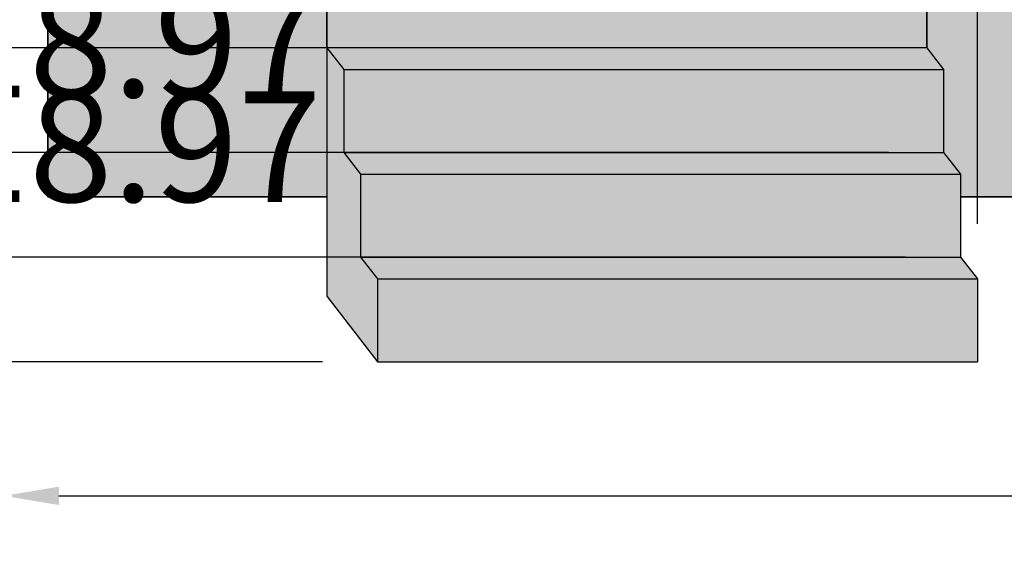
# Model space of a CAD drawing. Units: millimetres. Extents: x 130 to 1021, y 147 to 699.
# Tile 2 of 40: x 302 to 481, y 147 to 246. Entities that reach past the tile are written whole.
import ezdxf

# ---------------------------------------------------------------- set-up
doc = ezdxf.new("R2010")
doc.units = ezdxf.units.MM
doc.header["$MEASUREMENT"] = 0
for name, color, linetype, lineweight in [('A-ANNO-DIMS', 2, 'Continuous', 18), ('A-ELEV', 7, 'Continuous', 35), ('A-ELEV-PATT', 9, 'Continuous', 13), ('A-FLOR-STRS', 2, 'Continuous', 25)]:
    doc.layers.add(name, color=color, linetype=linetype, lineweight=lineweight)
doc.styles.get("Standard").update_dxf_attribs({"font": 'arial.ttf'})
doc.dimstyles.get("Standard").update_dxf_attribs({"dimtxt": 20, "dimasz": 10, "dimexe": 10, "dimexo": 10, "dimgap": 5, "dimtad": 0, "dimtih": 1, "dimtoh": 1, "dimdec": 0, "dimzin": 0, "dimdsep": 46, "dimtxsty": 'Standard', "dimcen": 5, "dimadec": 0, "dimazin": 0, "dimtfac": 1, "dimtdec": 0, "dimtofl": 0, "dimtmove": 0, "dimatfit": 3, "dimfxl": 1, "dimtolj": 1, "dimtzin": 0, "dimarcsym": 0})

# ---------------------------------------------------------------- blocks, each defined once
blk = doc.blocks.new('*D10')
at = {"layer": 'A-ANNO-DIMS', "color": 0, "lineweight": -2, "transparency": 16777216}
for p, q in [((440.89, 273.72), (430.89, 273.71)), ((473.57, 273.75), (483.57, 273.75)), ((450.9, 267.56), (450.9, 263.73)), ((463.58, 267.57), (463.58, 263.74))]:
    blk.add_line(p, q, dxfattribs=at)
at = {"layer": 'A-ANNO-DIMS', "color": 0, "transparency": 16777216}
for points in [[(440.89, 275.38), (440.89, 272.05), (450.89, 273.73)], [(473.57, 275.41), (473.58, 272.08), (463.57, 273.74)]]:
    blk.add_solid(points, dxfattribs=at)
at = {"layer": 'Defpoints', "color": 0, "transparency": 16777216}
for p in [(450.89, 277.56), (463.57, 277.57), (463.57, 273.74)]:
    blk.add_point(p, dxfattribs=at)
at = {"layer": 'A-ANNO-DIMS', "color": 0, "transparency": 16777216, "insert": (536.31, 273.75), "char_height": 20, "attachment_point": 5}
blk.add_mtext('\\A1;13 TYP.', dxfattribs=at)
blk = doc.blocks.new('*D11')
at = {"layer": 'A-ANNO-DIMS', "color": 0, "lineweight": -2, "transparency": 16777216}
for p, q in [((737.37, 648.7), (737.37, 149.74)), ((299.37, 566.95), (299.37, 149.74)), ((309.37, 159.74), (490.86, 159.74)), ((727.37, 159.74), (545.89, 159.74))]:
    blk.add_line(p, q, dxfattribs=at)
at = {"layer": 'A-ANNO-DIMS', "color": 0, "transparency": 16777216}
for points in [[(309.37, 161.41), (309.37, 158.07), (299.37, 159.74)], [(727.37, 161.41), (727.37, 158.07), (737.37, 159.74)]]:
    blk.add_solid(points, dxfattribs=at)
at = {"layer": 'Defpoints', "color": 0, "transparency": 16777216}
for p in [(737.37, 658.7), (299.37, 576.95), (737.37, 159.74)]:
    blk.add_point(p, dxfattribs=at)
at = {"layer": 'A-ANNO-DIMS', "color": 0, "transparency": 16777216, "insert": (518.37, 159.74), "char_height": 20, "attachment_point": 5}
blk.add_mtext('\\A1;438', dxfattribs=at)
blk = doc.blocks.new('*D12')
at = {"layer": 'A-ANNO-DIMS', "color": 0, "lineweight": -2, "transparency": 16777216}
for p, q in [((477.37, 661.95), (265.07, 661.95)), ((275.07, 651.95), (275.07, 438.2)), ((275.07, 194.04), (275.07, 407.78)), ((357.16, 184.04), (265.07, 184.04))]:
    blk.add_line(p, q, dxfattribs=at)
at = {"layer": 'A-ANNO-DIMS', "color": 0, "transparency": 16777216}
for points in [[(273.41, 651.95), (276.74, 651.95), (275.07, 661.95)], [(273.41, 194.04), (276.74, 194.04), (275.07, 184.04)]]:
    blk.add_solid(points, dxfattribs=at)
at = {"layer": 'Defpoints', "color": 0, "transparency": 16777216}
for p in [(275.07, 661.95), (487.37, 661.95), (367.16, 184.04)]:
    blk.add_point(p, dxfattribs=at)
at = {"layer": 'A-ANNO-DIMS', "color": 0, "transparency": 16777216, "insert": (275.07, 422.99), "char_height": 20, "attachment_point": 5}
blk.add_mtext('\\A1;477.9', dxfattribs=at)
blk = doc.blocks.new('*D23')
at = {"layer": 'A-ANNO-DIMS', "color": 0, "lineweight": -2, "transparency": 16777216}
for p, q in [((466.77, 403.95), (466.77, 696.25)), ((475.99, 209.04), (475.99, 696.25)), ((456.77, 686.25), (446.77, 686.25)), ((485.99, 686.25), (495.99, 686.25))]:
    blk.add_line(p, q, dxfattribs=at)
at = {"layer": 'A-ANNO-DIMS', "color": 0, "transparency": 16777216}
for points in [[(456.77, 687.91), (456.77, 684.58), (466.77, 686.25)], [(485.99, 687.91), (485.99, 684.58), (475.99, 686.25)]]:
    blk.add_solid(points, dxfattribs=at)
at = {"layer": 'Defpoints', "color": 0, "transparency": 16777216}
for p in [(475.99, 686.25), (466.77, 393.95), (475.99, 199.04)]:
    blk.add_point(p, dxfattribs=at)
at = {"layer": 'A-ANNO-DIMS', "color": 0, "transparency": 16777216, "insert": (534.63, 686.25), "char_height": 20, "attachment_point": 5}
blk.add_mtext('\\A1;9.222', dxfattribs=at)
blk = doc.blocks.new('*D24')
at = {"layer": 'A-ANNO-DIMS', "color": 0, "lineweight": -2, "transparency": 16777216}
for p, q in [((475.99, 209.04), (475.99, 696.25)), ((487.37, 671.95), (487.37, 696.25)), ((465.99, 686.25), (455.99, 686.25)), ((497.37, 686.25), (507.37, 686.25))]:
    blk.add_line(p, q, dxfattribs=at)
at = {"layer": 'A-ANNO-DIMS', "color": 0, "transparency": 16777216}
for points in [[(465.99, 687.91), (465.99, 684.58), (475.99, 686.25)], [(497.37, 687.91), (497.37, 684.58), (487.37, 686.25)]]:
    blk.add_solid(points, dxfattribs=at)
at = {"layer": 'Defpoints', "color": 0, "transparency": 16777216}
for p in [(487.37, 686.25), (487.37, 661.95), (475.99, 199.04)]:
    blk.add_point(p, dxfattribs=at)
at = {"layer": 'A-ANNO-DIMS', "color": 0, "transparency": 16777216, "insert": (553.02, 686.25), "char_height": 20, "attachment_point": 5}
blk.add_mtext('\\A1;11.385', dxfattribs=at)
blk = doc.blocks.new('*D33')
at = {"layer": 'A-ANNO-DIMS', "color": 0, "lineweight": -2, "transparency": 16777216}
for p, q in [((275.07, 213.01), (275.07, 223.01)), ((275.07, 223.01), (285.07, 223.01)), ((462.91, 203.01), (265.07, 203.01)), ((357.16, 184.04), (265.07, 184.04)), ((275.07, 174.04), (275.07, 164.04))]:
    blk.add_line(p, q, dxfattribs=at)
at = {"layer": 'A-ANNO-DIMS', "color": 0, "transparency": 16777216}
for points in [[(273.41, 213.01), (276.74, 213.01), (275.07, 203.01)], [(273.41, 174.04), (276.74, 174.04), (275.07, 184.04)]]:
    blk.add_solid(points, dxfattribs=at)
at = {"layer": 'Defpoints', "color": 0, "transparency": 16777216}
for p in [(275.07, 203.01), (472.91, 203.01), (367.16, 184.04)]:
    blk.add_point(p, dxfattribs=at)
at = {"layer": 'A-ANNO-DIMS', "color": 0, "transparency": 16777216, "insert": (322.88, 223.01), "char_height": 20, "attachment_point": 5}
blk.add_mtext('\\A1;18.97', dxfattribs=at)
blk = doc.blocks.new('*D34')
at = {"layer": 'A-ANNO-DIMS', "color": 0, "lineweight": -2, "transparency": 16777216}
for p, q in [((275.07, 231.98), (275.07, 241.98)), ((275.07, 241.98), (285.07, 241.98)), ((459.84, 221.98), (265.07, 221.98)), ((462.91, 203.01), (265.07, 203.01)), ((275.07, 193.01), (275.07, 183.01))]:
    blk.add_line(p, q, dxfattribs=at)
at = {"layer": 'A-ANNO-DIMS', "color": 0, "transparency": 16777216}
for points in [[(273.41, 231.98), (276.74, 231.98), (275.07, 221.98)], [(273.41, 193.01), (276.74, 193.01), (275.07, 203.01)]]:
    blk.add_solid(points, dxfattribs=at)
at = {"layer": 'Defpoints', "color": 0, "transparency": 16777216}
for p in [(275.07, 221.98), (469.84, 221.98), (472.91, 203.01)]:
    blk.add_point(p, dxfattribs=at)
at = {"layer": 'A-ANNO-DIMS', "color": 0, "transparency": 16777216, "insert": (322.88, 241.98), "char_height": 20, "attachment_point": 5}
blk.add_mtext('\\A1;18.97', dxfattribs=at)
blk = doc.blocks.new('*D35')
at = {"layer": 'A-ANNO-DIMS', "color": 0, "lineweight": -2, "transparency": 16777216}
for p, q in [((275.07, 250.95), (275.07, 260.95)), ((275.07, 260.95), (285.07, 260.95)), ((456.77, 240.95), (265.07, 240.95)), ((459.84, 221.98), (265.07, 221.98)), ((275.07, 211.98), (275.07, 201.98))]:
    blk.add_line(p, q, dxfattribs=at)
at = {"layer": 'A-ANNO-DIMS', "color": 0, "transparency": 16777216}
for points in [[(273.41, 250.95), (276.74, 250.95), (275.07, 240.95)], [(273.41, 211.98), (276.74, 211.98), (275.07, 221.98)]]:
    blk.add_solid(points, dxfattribs=at)
at = {"layer": 'Defpoints', "color": 0, "transparency": 16777216}
for p in [(275.07, 240.95), (466.77, 240.95), (469.84, 221.98)]:
    blk.add_point(p, dxfattribs=at)
at = {"layer": 'A-ANNO-DIMS', "color": 0, "transparency": 16777216, "insert": (322.88, 260.95), "char_height": 20, "attachment_point": 5}
blk.add_mtext('\\A1;18.97', dxfattribs=at)
blk = doc.blocks.new('*D36')
at = {"layer": 'A-ANNO-DIMS', "color": 0, "lineweight": -2, "transparency": 16777216}
for p, q in [((275.07, 270.95), (275.07, 280.95)), ((275.07, 280.95), (285.07, 280.95)), ((297.37, 260.95), (265.07, 260.95)), ((456.77, 240.95), (265.07, 240.95)), ((275.07, 230.95), (275.07, 220.95))]:
    blk.add_line(p, q, dxfattribs=at)
at = {"layer": 'A-ANNO-DIMS', "color": 0, "transparency": 16777216}
for points in [[(273.41, 270.95), (276.74, 270.95), (275.07, 260.95)], [(273.41, 230.95), (276.74, 230.95), (275.07, 240.95)]]:
    blk.add_solid(points, dxfattribs=at)
at = {"layer": 'Defpoints', "color": 0, "transparency": 16777216}
for p in [(275.07, 260.95), (307.37, 260.95), (466.77, 240.95)]:
    blk.add_point(p, dxfattribs=at)
at = {"layer": 'A-ANNO-DIMS', "color": 0, "transparency": 16777216, "insert": (304.53, 280.95), "char_height": 20, "attachment_point": 5}
blk.add_mtext('\\A1;20', dxfattribs=at)
blk = doc.blocks.new('*D37')
at = {"layer": 'A-ANNO-DIMS', "color": 0, "lineweight": -2, "transparency": 16777216}
for p, q in [((275.07, 283.95), (275.07, 293.95)), ((275.07, 293.95), (285.07, 293.95)), ((297.37, 273.95), (265.07, 273.95)), ((297.37, 260.95), (265.07, 260.95)), ((275.07, 250.95), (275.07, 240.95))]:
    blk.add_line(p, q, dxfattribs=at)
at = {"layer": 'A-ANNO-DIMS', "color": 0, "transparency": 16777216}
for points in [[(273.41, 283.95), (276.74, 283.95), (275.07, 273.95)], [(273.41, 250.95), (276.74, 250.95), (275.07, 260.95)]]:
    blk.add_solid(points, dxfattribs=at)
at = {"layer": 'Defpoints', "color": 0, "transparency": 16777216}
for p in [(275.07, 273.95), (307.37, 273.95), (307.37, 260.95)]:
    blk.add_point(p, dxfattribs=at)
at = {"layer": 'A-ANNO-DIMS', "color": 0, "transparency": 16777216, "insert": (303.46, 293.95), "char_height": 20, "attachment_point": 5}
blk.add_mtext('\\A1;13', dxfattribs=at)

msp = doc.modelspace()

# ---------------------------------------------------------------- hatches: boundary and pattern name
at = {"layer": 'A-ELEV-PATT'}
h = msp.add_hatch(color=256, dxfattribs=at)
h.dxf.hatch_style = 1
h.paths.add_polyline_path([(737.3738, 658.6988, 0.01359606), (632.4019, 661.9473), (607.3738, 661.9473), (487.3738, 661.9473), (487.3738, 649.9473), (607.3738, 649.9473), (632.3794, 649.9473, -0.01368411), (737.3738, 646.6784)])
h.paths.add_polyline_path([(732.3738, 643.9599, 0.01305286), (632.3738, 646.9473), (607.3738, 646.9473), (487.3738, 646.9473), (487.3738, 596.9473), (632.3738, 596.9473, -0.01305286), (732.3738, 593.9599)])
h.paths.add_polyline_path([(737.3738, 593.6732, 0.01370629), (632.3738, 596.9473), (487.3738, 596.9473), (487.3738, 586.9473), (632.355, 586.9473, -0.01378075), (737.3738, 583.6559)])
h.paths.add_polyline_path([(447.3738, 646.9473), (307.3738, 646.9473), (302.3738, 646.9473), (302.3738, 634.9473), (447.3738, 634.9473)])
h.paths.add_polyline_path([(447.3738, 631.9473), (307.3738, 631.9473), (307.3738, 586.9473), (447.3738, 586.9473)])
h.paths.add_polyline_path([(447.3738, 586.9473), (307.3738, 586.9473), (302.3738, 586.9473), (302.3738, 576.9473), (447.3738, 576.9473)])
h.paths.add_polyline_path([(447.3738, 573.9473), (367.3738, 573.9473), (367.3738, 539.9473), (447.3738, 539.9473)])
h.paths.add_polyline_path([(447.3738, 537.9473), (367.3738, 537.9473), (367.3738, 507.9473), (400.392, 507.4253, -0.00172798), (401.3281, 507.6451, -0.52200255), (425.6117, 511.0391, -0.03918489), (447.3738, 510.4359), (447.3738, 510.7883)])
h.paths.add_polyline_path([(394.7238, 505.9473), (367.3738, 505.9473), (367.3738, 476.9473, -0.0146512), (375.8501, 480.2159), (376.1506, 499.2266, -0.03554194)])
h.paths.add_polyline_path([(632.3738, 583.9473), (552.3738, 583.9473), (552.3738, 550.9473), (632.3738, 550.9473)])
h.paths.add_polyline_path([(632.3738, 548.9473), (552.3738, 548.9473), (552.3738, 515.9473), (632.3738, 515.9473)])
h.paths.add_polyline_path([(632.3738, 513.9473), (552.3738, 513.9473), (552.3738, 476.9473), (632.3738, 476.9473)])
h.paths.add_polyline_path([(737.3738, 473.6903, 0.01363261), (632.3926, 476.9473), (552.3738, 476.9473), (487.3738, 476.9473), (487.3738, 466.9473), (632.3738, 466.9473, -0.01370629), (737.3738, 463.6732)])
h.paths.add_polyline_path([(732.3738, 460.9552, 0.01307409), (632.3681, 463.9473), (487.3738, 463.9473), (487.3738, 407.735, -0.00322862), (489.3544, 406.9473), (632.3926, 406.9473, -0.01298259), (732.3738, 403.9755)])
h.paths.add_polyline_path([(487.3738, 463.9473, 0.20132998), (367.3738, 463.9473), (367.3738, 407.735, -0.18820307), (487.3738, 407.735)])
h.paths.add_polyline_path([(367.3738, 476.9473), (367.3738, 466.9473, -0.20133085), (487.3738, 466.9473), (487.3738, 476.9473, 0.20132998)])
h.paths.add_polyline_path([(367.3738, 463.9473), (307.3738, 463.9473), (307.3738, 401.9473), (357.9413, 401.9473), (367.3738, 407.735)])
h.paths.add_polyline_path([(367.3738, 476.9473), (302.3738, 476.9473), (302.3738, 466.9473), (367.3738, 466.9473)])
h.paths.add_polyline_path([(632.8184, 366.9453), (552.3738, 366.9453), (552.3738, 393.9473), (632.8184, 393.9473)])
h.paths.add_polyline_path([(632.8184, 357.2114), (632.8184, 363.9453), (552.3738, 363.9453), (552.3738, 357.2114), (552.3738, 336.9453), (632.8184, 336.9453)])
h.paths.add_polyline_path([(632.8184, 333.9453), (552.3738, 333.9453), (552.3738, 306.9453), (632.8184, 306.9453)])
h.paths.add_polyline_path([(632.8184, 303.9453), (552.3738, 303.9453), (552.3738, 273.9473), (632.355, 273.9473, 0.00006077), (632.8184, 273.9491)])
h.paths.add_polyline_path([(737.3738, 403.6903, 0.01363261), (632.3926, 406.9473), (489.3544, 406.9473, 0.19154808), (367.3738, 407.735), (367.3738, 396.9473, -0.20133085), (487.3738, 396.9473), (632.3738, 396.9473, -0.01370629), (737.3738, 393.6732)])
h.paths.add_polyline_path([(357.9413, 401.9473), (307.3738, 401.9473), (307.3738, 391.9473), (357.9413, 391.9473)])
h.paths.add_polyline_path([(357.9413, 357.2114), (357.9413, 388.9473), (307.3738, 388.9473), (307.3738, 357.2114), (307.3738, 273.9473), (357.9413, 273.9473)])
h.paths.add_polyline_path([(732.3738, 263.93, -0.0130317), (632.3794, 260.9473), (466.7667, 260.9473), (466.7667, 240.9473), (469.8406, 236.978), (469.8406, 221.978), (472.9145, 218.0087), (472.9145, 213.9473), (607.3738, 213.9473), (732.3738, 213.9473)])
h.paths.add_polyline_path([(732.3738, 290.889), (722.479, 290.889), (722.479, 301.889), (732.3738, 301.889), (732.3738, 305.889), (722.479, 305.889), (722.479, 316.889), (732.3738, 316.889), (732.3738, 320.889), (722.479, 320.889), (722.479, 331.889), (732.3738, 331.889), (732.3738, 335.889), (722.479, 335.889), (722.479, 346.889), (732.3738, 346.889), (732.3738, 350.889), (722.479, 350.889), (722.479, 361.889), (732.3738, 361.889), (732.3738, 365.889), (722.479, 365.889), (722.479, 376.889), (732.3738, 376.889), (732.3738, 380.889), (722.479, 380.889), (722.479, 391.4848, 0.00052326), (718.479, 391.6843), (718.479, 380.889), (707.479, 380.889), (707.479, 392.1896, 0.00052307), (703.479, 392.3576), (703.479, 380.889), (692.479, 380.889), (692.479, 392.7765, 0.00052292), (688.479, 392.9131), (688.479, 380.889), (677.479, 380.889), (677.479, 393.2456, 0.00052279), (673.479, 393.3508), (673.479, 380.889), (662.479, 380.889), (662.479, 393.597, 0.0005227), (658.479, 393.6709), (658.479, 380.889), (647.479, 380.889), (647.479, 393.8308, 0.00052264), (643.479, 393.8732), (643.479, 380.889), (632.8184, 380.889), (632.8184, 376.889), (643.479, 376.889), (643.479, 365.889), (632.8184, 365.889), (632.8184, 361.889), (643.479, 361.889), (643.479, 350.889), (632.8184, 350.889), (632.8184, 346.889), (643.479, 346.889), (643.479, 335.889), (632.8184, 335.889), (632.8184, 331.889), (643.479, 331.889), (643.479, 320.889), (632.8184, 320.889), (632.8184, 316.889), (643.479, 316.889), (643.479, 305.889), (632.8184, 305.889), (632.8184, 301.889), (643.479, 301.889), (643.479, 290.889), (632.8184, 290.889), (632.8184, 286.889), (643.479, 286.889), (643.479, 274.0217, 0.00052456), (647.479, 274.0643), (647.479, 286.889), (658.479, 286.889), (658.479, 274.2248, 0.00052462), (662.479, 274.2989), (662.479, 286.889), (673.479, 286.889), (673.479, 274.546, 0.00052471), (677.479, 274.6516), (677.479, 286.889), (688.479, 286.889), (688.479, 274.9853, 0.00052484), (692.479, 275.1224), (692.479, 286.889), (703.479, 286.889), (703.479, 275.5429, 0.000525), (707.479, 275.7115), (707.479, 286.889), (718.479, 286.889), (718.479, 276.2187, 0.00052519), (722.479, 276.4189), (722.479, 286.889), (732.3738, 286.889)])
h.paths.add_polyline_path([(718.479, 290.889), (707.479, 290.889), (707.479, 301.889), (718.479, 301.889)], flags=16)
h.paths.add_polyline_path([(703.479, 290.889), (692.479, 290.889), (692.479, 301.889), (703.479, 301.889)], flags=16)
h.paths.add_polyline_path([(718.479, 305.889), (707.479, 305.889), (707.479, 316.889), (718.479, 316.889)], flags=16)
h.paths.add_polyline_path([(703.479, 305.889), (692.479, 305.889), (692.479, 316.889), (703.479, 316.889)], flags=16)
h.paths.add_polyline_path([(688.479, 290.889), (677.479, 290.889), (677.479, 301.889), (688.479, 301.889)], flags=16)
h.paths.add_polyline_path([(718.479, 320.889), (707.479, 320.889), (707.479, 331.889), (718.479, 331.889)], flags=16)
h.paths.add_polyline_path([(688.479, 305.889), (677.479, 305.889), (677.479, 316.889), (688.479, 316.889)], flags=16)
h.paths.add_polyline_path([(703.479, 320.889), (692.479, 320.889), (692.479, 331.889), (703.479, 331.889)], flags=16)
h.paths.add_polyline_path([(688.479, 320.889), (677.479, 320.889), (677.479, 331.889), (688.479, 331.889)], flags=16)
h.paths.add_polyline_path([(673.479, 290.889), (662.479, 290.889), (662.479, 301.889), (673.479, 301.889)], flags=16)
h.paths.add_polyline_path([(718.479, 335.889), (707.479, 335.889), (707.479, 346.889), (718.479, 346.889)], flags=16)
h.paths.add_polyline_path([(673.479, 305.889), (662.479, 305.889), (662.479, 316.889), (673.479, 316.889)], flags=16)
h.paths.add_polyline_path([(703.479, 335.889), (692.479, 335.889), (692.479, 346.889), (703.479, 346.889)], flags=16)
h.paths.add_polyline_path([(673.479, 320.889), (662.479, 320.889), (662.479, 331.889), (673.479, 331.889)], flags=16)
h.paths.add_polyline_path([(688.479, 335.889), (677.479, 335.889), (677.479, 346.889), (688.479, 346.889)], flags=16)
h.paths.add_polyline_path([(658.479, 290.889), (647.479, 290.889), (647.479, 301.889), (658.479, 301.889)], flags=16)
h.paths.add_polyline_path([(718.479, 350.889), (707.479, 350.889), (707.479, 361.889), (718.479, 361.889)], flags=16)
h.paths.add_polyline_path([(658.479, 305.889), (647.479, 305.889), (647.479, 316.889), (658.479, 316.889)], flags=16)
h.paths.add_polyline_path([(703.479, 350.889), (692.479, 350.889), (692.479, 361.889), (703.479, 361.889)], flags=16)
h.paths.add_polyline_path([(673.479, 335.889), (662.479, 335.889), (662.479, 346.889), (673.479, 346.889)], flags=16)
h.paths.add_polyline_path([(658.479, 320.889), (647.479, 320.889), (647.479, 331.889), (658.479, 331.889)], flags=16)
h.paths.add_polyline_path([(688.479, 350.889), (677.479, 350.889), (677.479, 361.889), (688.479, 361.889)], flags=16)
h.paths.add_polyline_path([(718.479, 365.889), (707.479, 365.889), (707.479, 376.889), (718.479, 376.889)], flags=16)
h.paths.add_polyline_path([(658.479, 335.889), (647.479, 335.889), (647.479, 346.889), (658.479, 346.889)], flags=16)
h.paths.add_polyline_path([(673.479, 350.889), (662.479, 350.889), (662.479, 361.889), (673.479, 361.889)], flags=16)
h.paths.add_polyline_path([(703.479, 365.889), (692.479, 365.889), (692.479, 376.889), (703.479, 376.889)], flags=16)
h.paths.add_polyline_path([(688.479, 365.889), (677.479, 365.889), (677.479, 376.889), (688.479, 376.889)], flags=16)
h.paths.add_polyline_path([(658.479, 350.889), (647.479, 350.889), (647.479, 361.889), (658.479, 361.889)], flags=16)
h.paths.add_polyline_path([(673.479, 365.889), (662.479, 365.889), (662.479, 376.889), (673.479, 376.889)], flags=16)
h.paths.add_polyline_path([(658.479, 365.889), (647.479, 365.889), (647.479, 376.889), (658.479, 376.889)], flags=16)
h.paths.add_polyline_path([(732.3738, 503.9786), (722.3392, 503.9786), (722.3392, 514.9786), (732.3738, 514.9786), (732.3738, 518.9786), (722.3392, 518.9786), (722.3392, 529.9786), (732.3738, 529.9786), (732.3738, 533.9786), (722.3392, 533.9786), (722.3392, 544.9786), (732.3738, 544.9786), (732.3738, 546.9473), (732.3738, 548.9786), (722.3392, 548.9786), (722.3392, 559.9786), (732.3738, 559.9786), (732.3738, 563.9786), (722.3392, 563.9786), (722.3392, 574.9786), (732.3738, 574.9786), (732.3738, 578.9786), (722.3392, 578.9786), (722.3392, 581.4789, 0.00052601), (718.3392, 581.6791), (718.3392, 578.9786), (707.3392, 578.9786), (707.3392, 582.1863, 0.00052582), (703.3392, 582.355), (703.3392, 578.9786), (692.3392, 578.9786), (692.3392, 582.7752, 0.00052566), (688.3392, 582.9123), (688.3392, 578.9786), (677.3392, 578.9786), (677.3392, 583.2457, 0.00052554), (673.3392, 583.3512), (673.3392, 578.9786), (662.3392, 578.9786), (662.3392, 583.5978, 0.00052545), (658.3392, 583.6718), (658.3392, 578.9786), (647.3392, 578.9786), (647.3392, 583.8317, 0.00052539), (643.3392, 583.8741), (643.3392, 578.9786), (632.3738, 578.9786), (632.3738, 574.9786), (643.3392, 574.9786), (643.3392, 563.9786), (632.3738, 563.9786), (632.3738, 559.9786), (643.3392, 559.9786), (643.3392, 548.9786), (632.3738, 548.9786), (632.3738, 544.9786), (643.3392, 544.9786), (643.3392, 533.9786), (632.3738, 533.9786), (632.3738, 529.9786), (643.3392, 529.9786), (643.3392, 518.9786), (632.3738, 518.9786), (632.3738, 515.9473), (632.3738, 514.9786), (643.3392, 514.9786), (643.3392, 503.9786), (632.3738, 503.9786), (632.3738, 499.9786), (643.3392, 499.9786), (643.3392, 488.9786), (632.3738, 488.9786), (632.3738, 484.9786), (643.3392, 484.9786), (643.3392, 476.8751, -0.00051911), (647.3392, 476.8332), (647.3392, 484.9786), (658.3392, 484.9786), (658.3392, 476.6752, -0.00051917), (662.3392, 476.6022), (662.3392, 484.9786), (673.3392, 484.9786), (673.3392, 476.3585, -0.00051926), (677.3392, 476.2543), (677.3392, 484.9786), (688.3392, 484.9786), (688.3392, 475.9248, -0.00051938), (692.3392, 475.7894), (692.3392, 484.9786), (703.3392, 484.9786), (703.3392, 475.3741, -0.00051953), (707.3392, 475.2075), (707.3392, 484.9786), (718.3392, 484.9786), (718.3392, 474.7064, -0.00051972), (722.3392, 474.5086), (722.3392, 484.9786), (732.3738, 484.9786), (732.3738, 488.9786), (722.3392, 488.9786), (722.3392, 499.9786), (732.3738, 499.9786)])
h.paths.add_polyline_path([(718.3392, 503.9786), (707.3392, 503.9786), (707.3392, 514.9786), (718.3392, 514.9786)], flags=16)
h.paths.add_polyline_path([(718.3392, 499.9786), (718.3392, 488.9786), (707.3392, 488.9786), (707.3392, 499.9786)], flags=16)
h.paths.add_polyline_path([(718.3392, 518.9786), (707.3392, 518.9786), (707.3392, 529.9786), (718.3392, 529.9786)], flags=16)
h.paths.add_polyline_path([(703.3392, 503.9786), (692.3392, 503.9786), (692.3392, 514.9786), (703.3392, 514.9786)], flags=16)
h.paths.add_polyline_path([(703.3392, 499.9786), (703.3392, 488.9786), (692.3392, 488.9786), (692.3392, 499.9786)], flags=16)
h.paths.add_polyline_path([(703.3392, 518.9786), (692.3392, 518.9786), (692.3392, 529.9786), (703.3392, 529.9786)], flags=16)
h.paths.add_polyline_path([(718.3392, 533.9786), (707.3392, 533.9786), (707.3392, 544.9786), (718.3392, 544.9786)], flags=16)
h.paths.add_polyline_path([(688.3392, 503.9786), (677.3392, 503.9786), (677.3392, 514.9786), (688.3392, 514.9786)], flags=16)
h.paths.add_polyline_path([(688.3392, 499.9786), (688.3392, 488.9786), (677.3392, 488.9786), (677.3392, 499.9786)], flags=16)
h.paths.add_polyline_path([(703.3392, 533.9786), (692.3392, 533.9786), (692.3392, 544.9786), (703.3392, 544.9786)], flags=16)
h.paths.add_polyline_path([(688.3392, 518.9786), (677.3392, 518.9786), (677.3392, 529.9786), (688.3392, 529.9786)], flags=16)
h.paths.add_polyline_path([(688.3392, 533.9786), (677.3392, 533.9786), (677.3392, 544.9786), (688.3392, 544.9786)], flags=16)
h.paths.add_polyline_path([(718.3392, 548.9786), (707.3392, 548.9786), (707.3392, 559.9786), (718.3392, 559.9786)], flags=16)
h.paths.add_polyline_path([(673.3392, 503.9786), (662.3392, 503.9786), (662.3392, 514.9786), (673.3392, 514.9786)], flags=16)
h.paths.add_polyline_path([(673.3392, 499.9786), (673.3392, 488.9786), (662.3392, 488.9786), (662.3392, 499.9786)], flags=16)
h.paths.add_polyline_path([(703.3392, 548.9786), (692.3392, 548.9786), (692.3392, 559.9786), (703.3392, 559.9786)], flags=16)
h.paths.add_polyline_path([(673.3392, 518.9786), (662.3392, 518.9786), (662.3392, 529.9786), (673.3392, 529.9786)], flags=16)
h.paths.add_polyline_path([(688.3392, 548.9786), (677.3392, 548.9786), (677.3392, 559.9786), (688.3392, 559.9786)], flags=16)
h.paths.add_polyline_path([(673.3392, 533.9786), (662.3392, 533.9786), (662.3392, 544.9786), (673.3392, 544.9786)], flags=16)
h.paths.add_polyline_path([(718.3392, 563.9786), (707.3392, 563.9786), (707.3392, 574.9786), (718.3392, 574.9786)], flags=16)
h.paths.add_polyline_path([(658.3392, 503.9786), (647.3392, 503.9786), (647.3392, 514.9786), (658.3392, 514.9786)], flags=16)
h.paths.add_polyline_path([(658.3392, 499.9786), (658.3392, 488.9786), (647.3392, 488.9786), (647.3392, 499.9786)], flags=16)
h.paths.add_polyline_path([(703.3392, 563.9786), (692.3392, 563.9786), (692.3392, 574.9786), (703.3392, 574.9786)], flags=16)
h.paths.add_polyline_path([(658.3392, 518.9786), (647.3392, 518.9786), (647.3392, 529.9786), (658.3392, 529.9786)], flags=16)
h.paths.add_polyline_path([(673.3392, 548.9786), (662.3392, 548.9786), (662.3392, 559.9786), (673.3392, 559.9786)], flags=16)
h.paths.add_polyline_path([(688.3392, 563.9786), (677.3392, 563.9786), (677.3392, 574.9786), (688.3392, 574.9786)], flags=16)
h.paths.add_polyline_path([(658.3392, 533.9786), (647.3392, 533.9786), (647.3392, 544.9786), (658.3392, 544.9786)], flags=16)
h.paths.add_polyline_path([(673.3392, 563.9786), (662.3392, 563.9786), (662.3392, 574.9786), (673.3392, 574.9786)], flags=16)
h.paths.add_polyline_path([(658.3392, 548.9786), (647.3392, 548.9786), (647.3392, 559.9786), (658.3392, 559.9786)], flags=16)
h.paths.add_polyline_path([(658.3392, 563.9786), (647.3392, 563.9786), (647.3392, 574.9786), (658.3392, 574.9786)], flags=16)
h = msp.add_hatch(color=256, dxfattribs=at)
h.dxf.hatch_style = 1
h.paths.add_polyline_path([(364.0891, 218.0087), (361.0152, 221.978), (361.0152, 236.978), (357.9413, 240.9473), (357.9413, 195.9473), (367.163, 184.0395), (367.163, 199.0395), (364.0891, 203.0087)])
h.paths.add_polyline_path([(502.3738, 537.2685), (502.3738, 513.9473), (547.7773, 513.9473), (547.7773, 537.2685)])
h.paths.add_polyline_path([(502.3738, 511.9473), (502.3738, 481.7432), (547.7773, 481.7432), (547.7773, 511.9473)])
h.paths.add_polyline_path([(327.3738, 529.7), (327.3738, 509.9473), (363.922, 509.9473), (363.922, 529.7)])
h.paths.add_polyline_path([(327.3738, 507.9473), (327.3738, 480.95), (363.922, 480.95), (363.922, 507.9473)])
h = msp.add_hatch(color=256, dxfattribs=at)
h.dxf.hatch_style = 1
h.paths.add_polyline_path([(357.9413, 240.9473), (357.9413, 260.9473), (307.3738, 260.9473), (307.3738, 213.9473), (357.9413, 213.9473)])
h.paths.add_polyline_path([(382.3738, 260.9473), (357.9413, 260.9473), (357.9413, 240.9473), (466.7667, 240.9473), (466.7667, 260.9473), (432.3738, 260.9473), (432.3738, 249.5473), (382.3738, 249.5473)])
h.paths.add_polyline_path([(357.9413, 273.9473), (307.3738, 273.9473), (307.3738, 263.9473), (357.9413, 263.9473)])
h.paths.add_polyline_path([(382.3738, 273.9473), (357.9413, 273.9473), (357.9413, 263.9473), (382.3738, 263.9473)])
h = msp.add_hatch(color=256, dxfattribs=at)
h.dxf.hatch_style = 1
h.paths.add_polyline_path([(466.7667, 240.9473), (357.9413, 240.9473), (361.0152, 236.978), (469.8406, 236.978)])
h.paths.add_polyline_path([(472.9145, 218.0087), (469.8406, 221.978), (361.0152, 221.978), (364.0891, 218.0087)])
h.paths.add_polyline_path([(364.0891, 203.0087), (367.163, 199.0395), (475.9885, 199.0395), (472.9145, 203.0087)])
h = msp.add_hatch(color=256, dxfattribs=at)
h.dxf.hatch_style = 1
h.paths.add_polyline_path([(475.9885, 184.0395), (475.9885, 199.0395), (367.163, 199.0395), (367.163, 184.0395)])
h.paths.add_polyline_path([(472.9145, 203.0087), (472.9145, 218.0087), (364.0891, 218.0087), (364.0891, 203.0087)])
h.paths.add_polyline_path([(361.0152, 236.978), (361.0152, 221.978), (469.8406, 221.978), (469.8406, 236.978)])

# ---------------------------------------------------------------- linework, layer by layer
at = {"layer": 'A-ELEV'}
for p, q in [((307.3738, 357.2114), (307.3738, 213.9473)), ((357.9413, 273.9473), (357.9413, 240.9473)), ((466.7667, 260.9473), (466.7667, 240.9473)), ((307.3738, 213.9473), (357.9413, 213.9473)), ((472.9145, 213.9473), (607.3738, 213.9473))]:
    msp.add_line(p, q, dxfattribs=at)
at = {"layer": 'A-FLOR-STRS'}
for p, q in [((466.7667, 240.9473), (357.9413, 240.9473)), ((357.9413, 240.9473), (361.0152, 236.978)), ((357.9413, 240.9473), (357.9413, 195.9473)), ((466.7667, 240.9473), (469.8406, 236.978)), ((361.0152, 236.978), (361.0152, 221.978)), ((361.0152, 236.978), (469.8406, 236.978)), ((469.8406, 236.978), (469.8406, 221.978)), ((361.0152, 221.978), (364.0891, 218.0087)), ((361.0152, 221.978), (469.8406, 221.978)), ((469.8406, 221.978), (472.9145, 218.0087)), ((364.0891, 218.0087), (364.0891, 203.0087)), ((364.0891, 218.0087), (472.9145, 218.0087)), ((472.9145, 218.0087), (472.9145, 203.0087)), ((364.0891, 203.0087), (367.163, 199.0395)), ((364.0891, 203.0087), (472.9145, 203.0087)), ((472.9145, 203.0087), (475.9885, 199.0395)), ((367.163, 199.0395), (367.163, 184.0395)), ((367.163, 199.0395), (475.9885, 199.0395)), ((475.9885, 199.0395), (475.9885, 184.0395)), ((357.9413, 195.9473), (367.163, 184.0395)), ((367.163, 184.0395), (475.9885, 184.0395))]:
    msp.add_line(p, q, dxfattribs=at)

# ---------------------------------------------------------------- dimensions: what is measured, and where the dimension line sits
at = {"layer": 'A-ANNO-DIMS'}
for base, p1, p2, override, picture, middle in [((475.9885, 686.2473), (466.7667, 393.9473), (475.9885, 199.0395), {"dimdec": 3, "dimlfac": 1, "dimrnd": 0, "dimzin": 0, "dimdsep": 46, "dimlunit": 2}, '*D23', (534.631, 686.2473)), ((487.3738, 686.2473), (475.9885, 199.0395), (487.3738, 661.9473), {"dimdec": 3, "dimlfac": 1, "dimrnd": 0, "dimzin": 0, "dimdsep": 46, "dimlunit": 2}, '*D24', (553.0218, 686.2473)), ((737.3738, 159.7395), (299.3738, 576.9473), (737.3738, 658.6988), {"dimdec": 0, "dimlfac": 1, "dimrnd": 0, "dimzin": 0, "dimdsep": 46, "dimlunit": 2}, '*D11', (518.3738, 159.7395))]:
    dim = msp.add_linear_dim(base=base, p1=p1, p2=p2, dimstyle='Standard', override=override, dxfattribs=at)
    dim.commit()
    dim.dimension.update_dxf_attribs({"geometry": picture, "text_midpoint": middle})
for base, p1, p2, override, picture, middle in [((275.0738, 661.9473), (367.163, 184.0395), (487.3738, 661.9473), {"dimdec": 1, "dimlfac": 1, "dimrnd": 0, "dimzin": 0, "dimdsep": 46, "dimlunit": 2}, '*D12', (275.0738, 422.9934)), ((275.0738, 273.9473), (307.3738, 260.9473), (307.3738, 273.9473), {"dimdec": 0, "dimlfac": 1, "dimrnd": 0, "dimzin": 0, "dimdsep": 46, "dimlunit": 2}, '*D37', (303.4571, 293.9473)), ((275.0738, 260.9473), (466.7667, 240.9473), (307.3738, 260.9473), {"dimdec": 0, "dimlfac": 1, "dimrnd": 0, "dimzin": 0, "dimdsep": 46, "dimlunit": 2}, '*D36', (304.5349, 280.9473)), ((275.0738, 240.9473), (469.8406, 221.978), (466.7667, 240.9473), {"dimdec": 2, "dimlfac": 1, "dimrnd": 0, "dimzin": 0, "dimdsep": 46, "dimlunit": 2}, '*D35', (322.8773, 260.9473)), ((275.0738, 221.978), (472.9145, 203.0087), (469.8406, 221.978), {"dimdec": 2, "dimlfac": 1, "dimrnd": 0, "dimzin": 0, "dimdsep": 46, "dimlunit": 2}, '*D34', (322.8773, 241.978)), ((275.0738, 203.0087), (367.163, 184.0395), (472.9145, 203.0087), {"dimdec": 2, "dimlfac": 1, "dimrnd": 0, "dimzin": 0, "dimdsep": 46, "dimlunit": 2}, '*D33', (322.8773, 223.0087))]:
    dim = msp.add_linear_dim(base=base, p1=p1, p2=p2, angle=90, dimstyle='Standard', override=override, dxfattribs=at)
    dim.commit()
    dim.dimension.update_dxf_attribs({"geometry": picture, "text_midpoint": middle})
dim = msp.add_linear_dim(base=(463.5746, 273.7371), p1=(450.8885, 277.5595), p2=(463.5714, 277.5701), angle=0.047753, text='<> TYP.', dimstyle='Standard', override={"dimdec": 0, "dimrnd": 0, "dimzin": 0, "dimlunit": 2}, dxfattribs=at)
dim.commit()
dim.dimension.update_dxf_attribs({"geometry": '*D10', "text_midpoint": (536.3099, 273.7537)})

doc.saveas('drawing.dxf')
